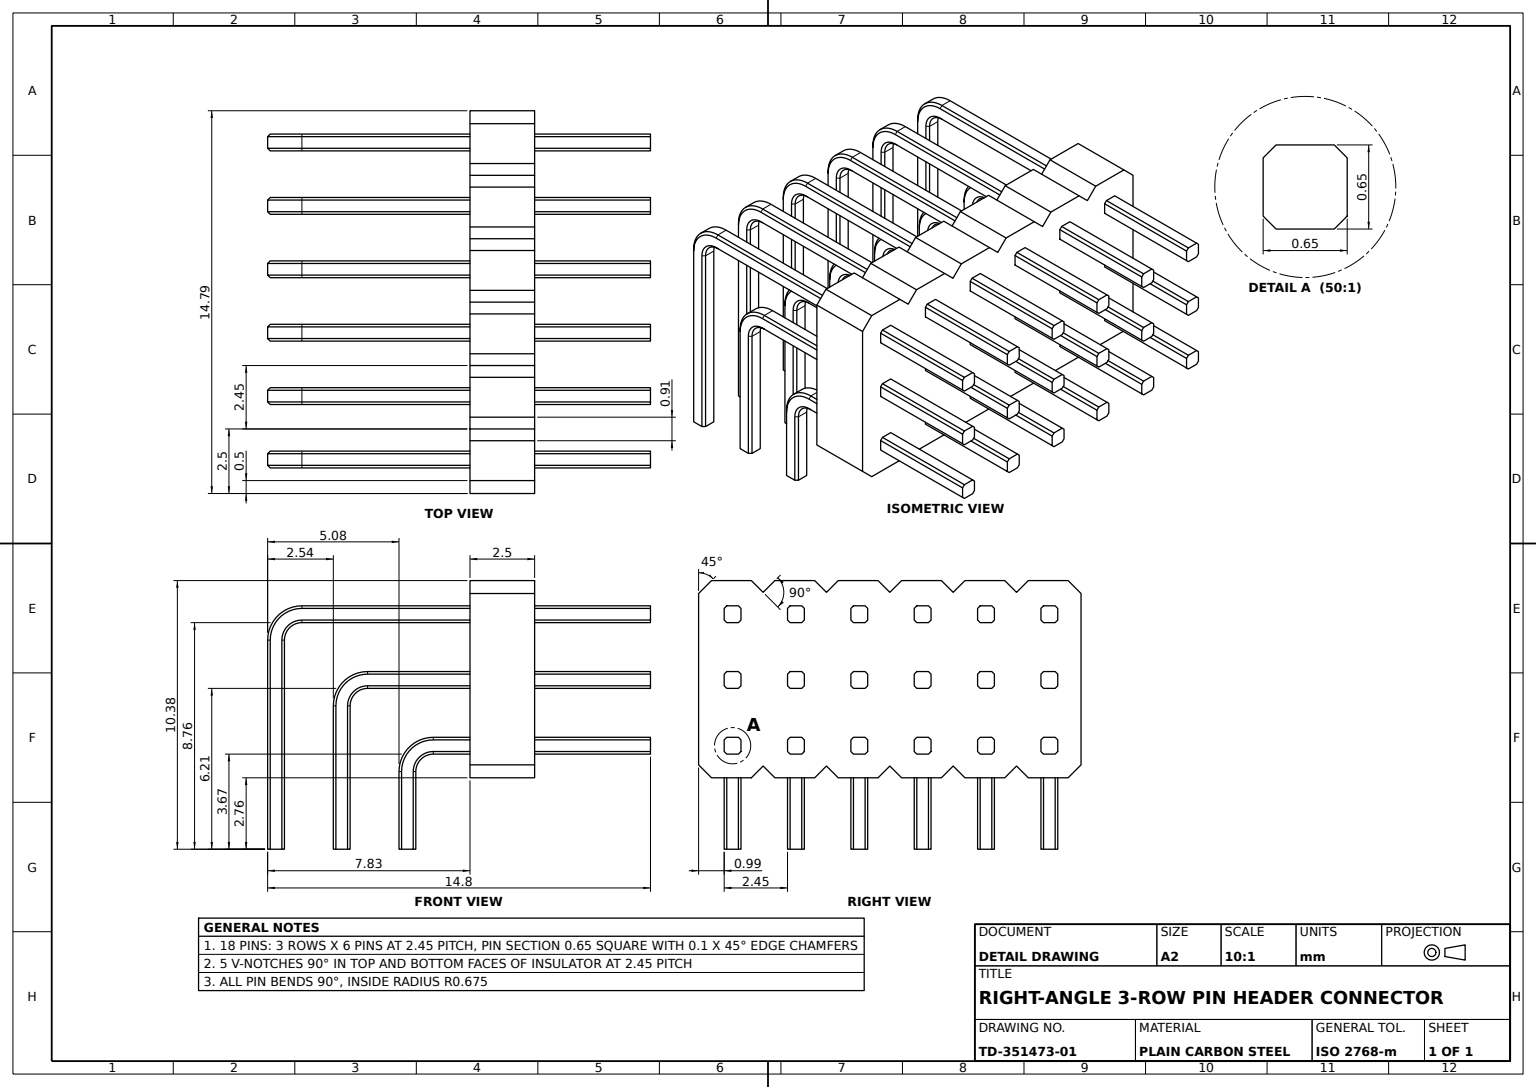
from build123d import *

# Parameters (mm, degrees)
INSULATOR_SEGMENT_DEPTH       = 2.5
PIN_POSITION_PATTERN_6X_COUNT = 6
PIN_POSITION_PATTERN_6X_PITCH = 2.45


with BuildPart() as part:
    # Pin Row 1 Sweep: sweep along a path in Pin Bend Path Sketch
    with BuildLine(Plane.XY) as pin_row_1_sweep_path:
        Line((5.08, 0), (5.08, 3))
        ThreePointArc((5.08, 3), (5.372893219, 3.707106781), (6.08, 4))
        Line((6.08, 4), (14.48, 4))
    # Pin Cross-Section Sketch → Pin Row 1 Sweep (sweep)
    with BuildSketch(Plane(origin=(0, 0, 0), x_dir=(1, 0, 0), z_dir=(0, 1, 0))):
        Polygon((4.855, 0.325), (5.305, 0.325), (5.405, 0.225), (5.405, -0.225), (5.305, -0.325), (4.855, -0.325), (4.755, -0.225), (4.755, 0.225), align=None)
    sweep(path=pin_row_1_sweep_path.line)



with BuildPart() as body_2:
    # Pin Row 2 Sweep: sweep along a path in Sketch2_3
    with BuildLine(Plane.XY) as pin_row_2_sweep_path:
        Line((2.54, 0), (2.54, 5.54))
        ThreePointArc((2.54, 5.54), (2.832893219, 6.247106781), (3.54, 6.54))
        Line((3.54, 6.54), (14.48, 6.54))
    # Sketch1_4 → Pin Row 2 Sweep (sweep)
    with BuildSketch(Plane(origin=(0, 0, 0), x_dir=(1, 0, 0), z_dir=(0, 1, 0))):
        Polygon((2.315, 0.325), (2.765, 0.325), (2.865, 0.225), (2.865, -0.225), (2.765, -0.325), (2.315, -0.325), (2.215, -0.225), (2.215, 0.225), align=None)
    sweep(path=pin_row_2_sweep_path.line)


with BuildPart() as body_3:
    # Pin Row 3 Sweep: sweep along a path in Sketch2_4
    with BuildLine(Plane.XY) as pin_row_3_sweep_path:
        Line((0, 0), (0, 8.08))
        ThreePointArc((0, 8.08), (0.292893219, 8.787106781), (1, 9.08))
        Line((1, 9.08), (14.48, 9.08))
    # Sketch1_5 → Pin Row 3 Sweep (sweep)
    with BuildSketch(Plane(origin=(0, 0, 0), x_dir=(1, 0, 0), z_dir=(0, 1, 0))):
        Polygon((-0.325, 0.225), (-0.225, 0.325), (0.225, 0.325), (0.325, 0.225), (0.325, -0.225), (0.225, -0.325), (-0.225, -0.325), (-0.325, -0.225), align=None)
    sweep(path=pin_row_3_sweep_path.line)


with BuildPart() as part_1:
    add(part.part)

    add(body_2.part)  # Insulator Segment merges body 2

    add(body_3.part)  # Insulator Segment merges body 3
    # Insulator Segment Sketch → Insulator Segment (add)
    with BuildSketch(Plane(origin=(7.5, 0, 0), x_dir=(0, 0, -1), z_dir=(1, 0, 0))):
        Polygon((-1.313948076, 9.879919797), (-0.813948076, 10.379919797), (0.726051924, 10.379919797), (1.226051924, 9.879919797), (1.226051924, 3.259919797), (0.726051924, 2.759919797), (-0.813948076, 2.759919797), (-1.313948076, 3.259919797), align=None)
    extrude(amount=INSULATOR_SEGMENT_DEPTH)


with BuildPart() as pin_position_pattern_6x_1:
    # Pin Position Pattern 6x: pattern copy
    add(part_1.part.moved(Location(Vector(0, 0, 1) * (1 * PIN_POSITION_PATTERN_6X_PITCH))))


with BuildPart() as pin_position_pattern_6x_2:
    # Pin Position Pattern 6x: pattern copy
    add(part_1.part.moved(Location(Vector(0, 0, 1) * (2 * PIN_POSITION_PATTERN_6X_PITCH))))


with BuildPart() as pin_position_pattern_6x_3:
    # Pin Position Pattern 6x: pattern copy
    add(part_1.part.moved(Location(Vector(0, 0, 1) * (3 * PIN_POSITION_PATTERN_6X_PITCH))))


with BuildPart() as pin_position_pattern_6x_4:
    # Pin Position Pattern 6x: pattern copy
    add(part_1.part.moved(Location(Vector(0, 0, 1) * (4 * PIN_POSITION_PATTERN_6X_PITCH))))


with BuildPart() as pin_position_pattern_6x_5:
    # Pin Position Pattern 6x: pattern copy
    add(part_1.part.moved(Location(Vector(0, 0, 1) * (5 * PIN_POSITION_PATTERN_6X_PITCH))))

    # Combine Header Body: union Pin Position Pattern 6x_4, Pin Position Pattern 6x_3, Pin Position Pattern 6x_2, Pin Position Pattern 6x_1, part
    add(pin_position_pattern_6x_4.part)
    add(pin_position_pattern_6x_3.part)
    add(pin_position_pattern_6x_2.part)
    add(pin_position_pattern_6x_1.part)
    add(part_1.part)


solid = pin_position_pattern_6x_5.part
